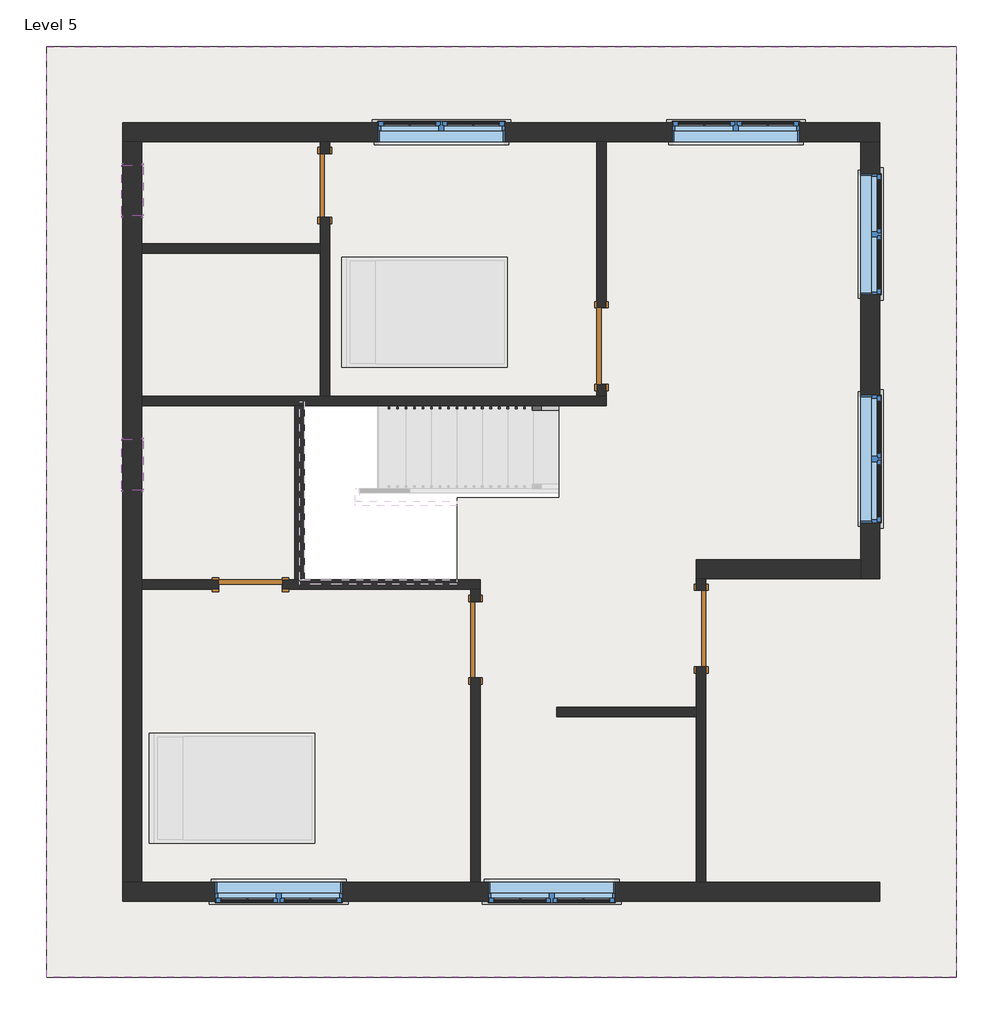
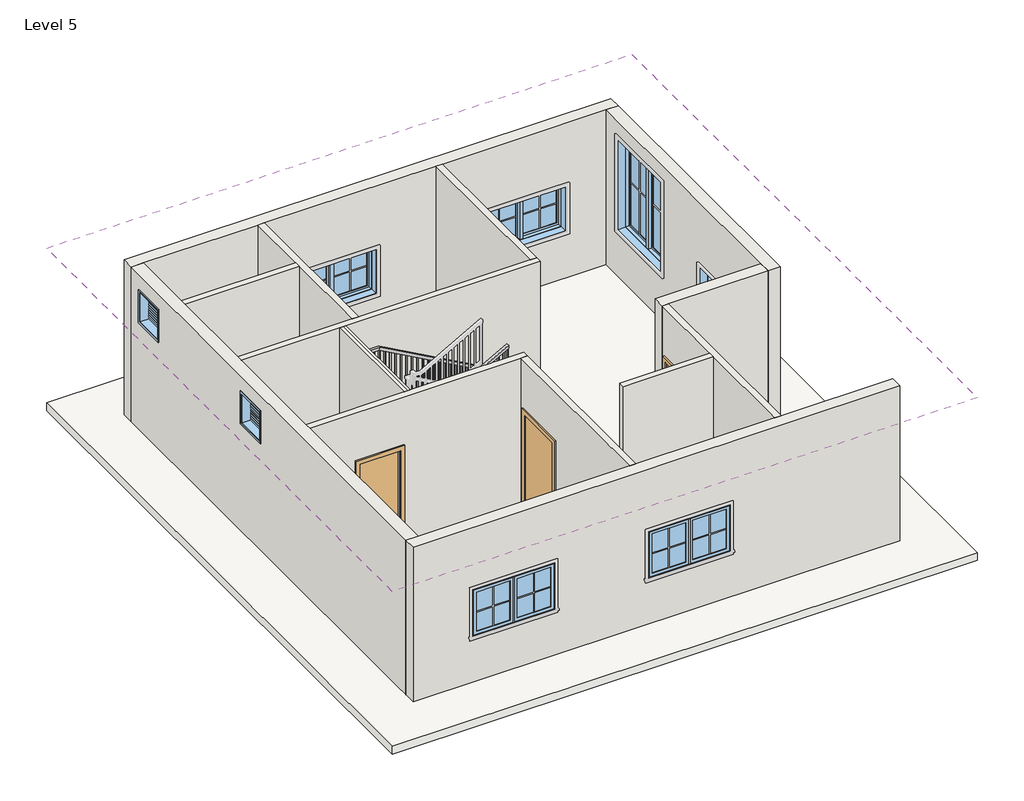
# One storey, part 1 of 2: 14 walls, 8 windows, 5 doors, 2 roofs, 1 railing.
# Revit data of these elements (continued)
# Elements 18, 19, 21, 22 (IfcWall, "WALL 9\"") (continued)
#   Top Offset = 0' - 0"
#   Base Offset = 0' - 0"
#   Unconnected Height = 10' - 0"
#   wall height = 10' - 0"
#   Phase Created = New Construction
#   Base Constraint = Level 5
#   Materials on its faces: "Default Wall", "Wood - Stained"
# Element 20 (IfcWall, "WALL 9\"")
#   Top Offset = 0' - 0"
#   Base Offset = 0' - 0"
#   Unconnected Height = 10' - 0"
#   wall height = 10' - 0"
#   Phase Created = New Construction
#   Base Constraint = Level 5
#   Materials on its faces: "Wood - Stained", "Default Wall"
# Element 23 (IfcWindow, "Window-Casement-Double : 57\" x 72\"")
#   Mark = "40"
#   Window Inset = 0' - 0"
#   Interior Wall Closure = 0' - 2 1/4"
#   Frame Extension = 0' - 0 1/4"
#   Exterior Wall Closure = 0' - 1 1/4"
#   Interior Trim Visibility = yes
#   Exterior Trim Visibility = yes
#   Phase Created = New Construction
#   Materials on its faces: "Wood - Stained", "Glass", "Clad - White"
# Element 24 (IfcWindow, "Window-Casement-Double : WINDOW 6\"")
#   Mark = "33"
#   Window Inset = 0' - 0"
#   Interior Wall Closure = 0' - 2 1/4"
#   Frame Extension = 0' - 0 1/4"
#   Exterior Wall Closure = 0' - 1 1/4"
#   Interior Trim Visibility = yes
#   Exterior Trim Visibility = yes
#   Phase Created = New Construction
#   Materials on its faces: "Wood - Stained", "Glass", "Clad - White"
# Element 25 (IfcWindow, "Window-Casement-Double : WINDOW 6\"")
#   Mark = "34"
#   Window Inset = 0' - 0"
#   Interior Wall Closure = 0' - 2 1/4"
#   Frame Extension = 0' - 0 1/4"
#   Exterior Wall Closure = 0' - 1 1/4"
#   Interior Trim Visibility = yes
#   Exterior Trim Visibility = yes
#   Phase Created = New Construction
#   Materials on its faces: "Wood - Stained", "Glass", "Clad - White"
# Element 26 (IfcWindow, "Window-Casement-Double : WINDOW 6\"")
#   Mark = "35"
#   Window Inset = 0' - 0"
#   Interior Wall Closure = 0' - 2 1/4"
#   Frame Extension = 0' - 0 1/4"
#   Exterior Wall Closure = 0' - 1 1/4"
#   Interior Trim Visibility = yes
#   Exterior Trim Visibility = yes
#   Phase Created = New Construction
#   Materials on its faces: "Wood - Stained", "Glass", "Clad - White"
# Element 27 (IfcWindow, "Window-Casement-Double : WINDOW 6\"")
#   Mark = "36"
#   Window Inset = 0' - 0"
#   Interior Wall Closure = 0' - 2 1/4"
#   Frame Extension = 0' - 0 1/4"
#   Exterior Wall Closure = 0' - 1 1/4"
#   Interior Trim Visibility = yes
#   Exterior Trim Visibility = yes
#   Phase Created = New Construction
#   Materials on its faces: "Wood - Stained", "Glass", "Clad - White"
# Element 28 (IfcWindow, "Window-Casement-Double : WINDOW 6\"")
#   Mark = "37"
#   Window Inset = 0' - 0"
#   Interior Wall Closure = 0' - 2 1/4"
#   Frame Extension = 0' - 0 1/4"
#   Exterior Wall Closure = 0' - 1 1/4"
#   Interior Trim Visibility = yes
#   Exterior Trim Visibility = yes
#   Phase Created = New Construction
#   Materials on its faces: "Wood - Stained", "Glass", "Clad - White"
# Element 29 (IfcWindow, "Window-Louvers : 24\" x 24\"")
#   Mark = "38"
#   Blade Width = 1' - 10 1/2"
#   Phase Created = New Construction
#   Materials on its faces: "Birch"
# Element 30 (IfcWindow, "Window-Louvers : 24\" x 24\"")
#   Mark = "39"
#   Blade Width = 1' - 10 1/2"
#   Phase Created = New Construction
#   Materials on its faces: "Birch"
# Materials
#   "Door - Panel": class "Wood", colour RGB 210 159 95, transparency 0, Cost = 0
#   "Door - Frame": colour RGB 118 70 51, transparency 0, Cost = 0
#   "Wood - Stained": class "Wood", colour RGB 224 178 126, transparency 0, Cost = 0
#   "Glass": class "Glass", colour RGB 0 128 192, transparency 0.75, Description = "Soda Lime Glass", Cost = 0
#   "Clad - White": class "Wood", colour RGB 242 242 238, transparency 0, Cost = 0
#   "Birch": class "Wood", colour RGB 224 178 126, transparency 0, Description = "Betula Alleghaniensis", Cost = 0
#   "Default Wall": colour RGB 128 128 128, transparency 0, Cost = 0
